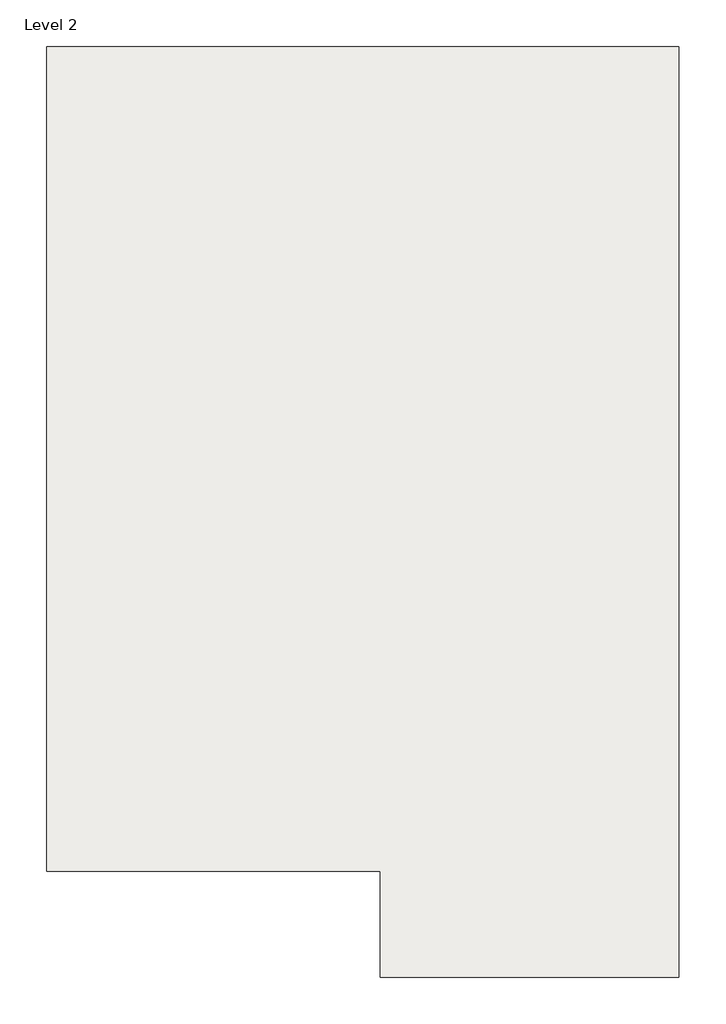
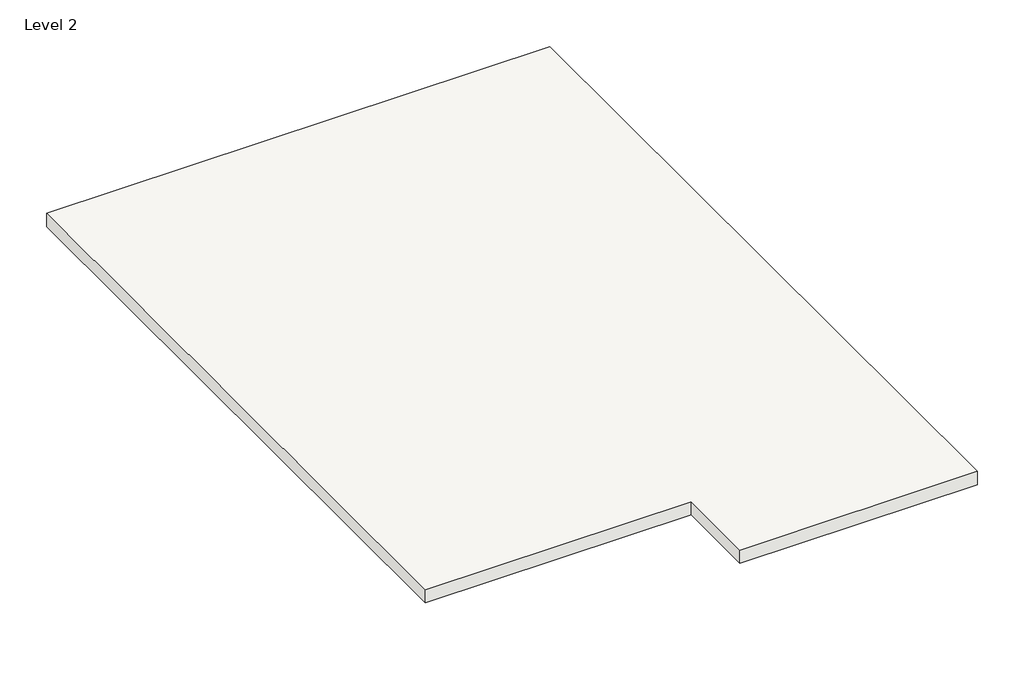
# One storey: 1 roof.
"""IFC4 building model written with IfcOpenShell, lengths in millimetres."""

from ifc_helpers import new_model, si_unit, frame, origin, place, context, project, spatial, polyline, outline, extrude, element, save

model = new_model("IFC4")

# Units and contexts
model_context = context("Model", 3, world=origin())
ifc_project = project(units=[si_unit("LENGTHUNIT", "METRE", prefix="MILLI")], contexts=[model_context])

# Site, building, storey
site = spatial("IfcSite", under=ifc_project)
building = spatial("IfcBuilding", under=site)
storey = spatial("IfcBuildingStorey", under=building, Name="Level 2", Elevation=3048.0)

# Roof
placement = place(None, origin())
element("IfcRoof", 1, ObjectType="Generic - 12\"", at=placement, inside=storey, context=model_context, shape_type="SweptSolid", body=[
    extrude(outline(polyline([(-11802.0976606, 14148.499435), (-930.8976606, 14148.499435), (-930.8976606, -1853.500565), (-6061.6976606, -1853.500565), (-6061.6976606, -24.700565), (-11802.0976606, -24.700565), (-11802.0976606, 14148.499435)])), frame((0.0, 0.0, 3048.0), z_axis=(0.0, 0.0, 1.0), x_axis=(1.0, 0.0, 0.0)), (0.0, 0.0, 1.0), 304.8),
])

save(model, "model.ifc")

# Revit data of these elements
# Type "Generic - 12\""
#   Assembly Code = "B1020"
#   Layers, outside or top first: 1' - 0" "Brick, Soldier Course" (function 1)
# Element 1 (IfcRoof, "Generic - 12\"")
#   built-in parameter 1001705 = 11 (stored number, unit not read)
#   built-in parameter 1001710 = 33615
#   Phase Created = New Construction
#   Materials on its faces: "Brick, Soldier Course"
# Materials
#   "Brick, Soldier Course": class "Masonry", colour RGB 170 98 104, transparency 0, Description = "Common brick soldier coursed", Cost = 0
